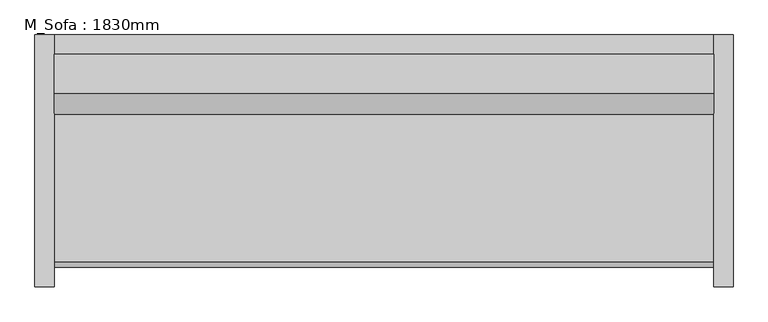
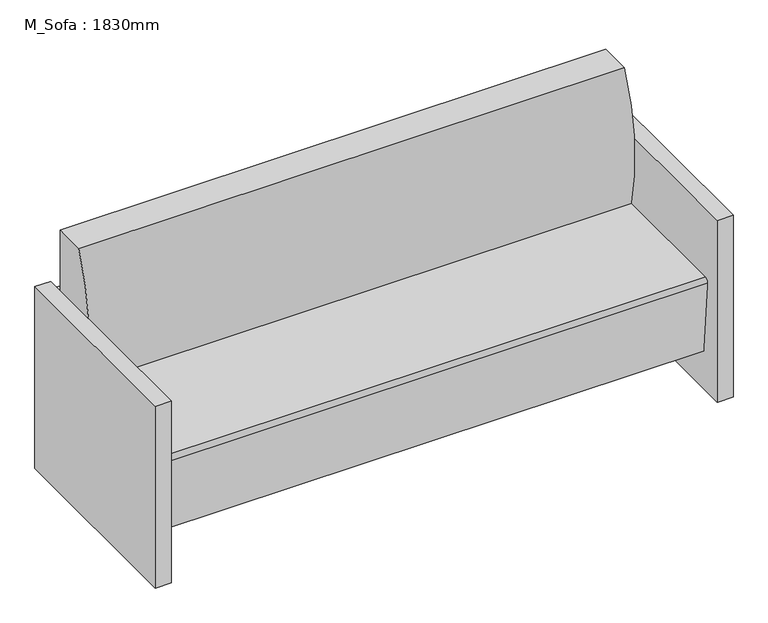
"""IFC4 building model written with IfcOpenShell, lengths in millimetres: furniture geometry, M_Sofa : 1830mm."""

from ifc_helpers import new_model, si_unit, point, frame, frame_2d, origin, origin_with_axes, place, context, project, spatial, polyline, circle_curve, trimmed, segment, composite_curve, outline, extrude, source, transform, mapped, element, save


def m_sofa_1830mm_f9e8a66b(model_context):
    return source(origin(), model_context, "Body", "SweptSolid", [
        extrude(outline(polyline([(-793.8295082, 425.5540984), (-793.8295082, 476.3540984), (934.5704918, 476.3540984), (934.5704918, 425.5540984), (-793.8295082, 425.5540984)])), frame((0.0, 0.0, 457.2), z_axis=(0.0, 0.0, 1.0), x_axis=(1.0, 0.0, 0.0)), (0.0, 0.0, 1.0), 127.0),
        extrude(outline(polyline([(-793.8295082, 425.5540984), (-793.8295082, 476.3540984), (934.5704918, 476.3540984), (934.5704918, 425.5540984), (-793.8295082, 425.5540984)])), frame((0.0, 0.0, 266.7), z_axis=(0.0, 0.0, 1.0), x_axis=(1.0, 0.0, 0.0)), (0.0, 0.0, 1.0), 127.0),
        extrude(outline(polyline([(-793.8295082, 425.5540984), (-793.8295082, 476.3540984), (934.5704918, 476.3540984), (934.5704918, 425.5540984), (-793.8295082, 425.5540984)])), frame((0.0, 0.0, 76.2), z_axis=(0.0, 0.0, 1.0), x_axis=(1.0, 0.0, 0.0)), (0.0, 0.0, 1.0), 127.0),
        extrude(outline(composite_curve([segment(trimmed(circle_curve(frame_2d((926.517198, 542.5300036)), 660.4), [point((286.1764935, 381.0))], [point((323.9540984, 812.8))], False, "CARTESIAN"), True, "CONTINUOUS"), segment(polyline([(323.9540984, 812.8), (425.5540984, 812.8), (425.5540984, 127.9665467), (-111.108343, 127.9665467), (-132.0379563, 367.1931221)]), True, "CONTINUOUS"), segment(trimmed(circle_curve(frame_2d((-119.3862837, 368.3)), 12.7), [point((-132.0379563, 367.1931221))], [point((-119.3862837, 381.0))], False, "CARTESIAN"), True, "CONTINUOUS"), segment(polyline([(-119.3862837, 381.0), (286.1764935, 381.0)]), True, "CONTINUOUS")], self_intersect=False)), frame((-793.8295082, 0.0, 0.0), z_axis=(1.0, 0.0, 0.0), x_axis=(0.0, 1.0, 0.0)), (0.0, 0.0, 1.0), 1728.4),
        extrude(outline(polyline([(-793.8295082, 476.3540984), (-793.8295082, -184.0459016), (-844.6295082, -184.0459016), (-844.6295082, 476.3540984), (-793.8295082, 476.3540984)])), origin_with_axes(), (0.0, 0.0, 1.0), 609.6),
        extrude(outline(polyline([(985.3704918, 476.3540984), (985.3704918, -184.0459016), (934.5704918, -184.0459016), (934.5704918, 476.3540984), (985.3704918, 476.3540984)])), origin_with_axes(), (0.0, 0.0, 1.0), 609.6),
    ])


if __name__ == "__main__":
    model = new_model("IFC4")
    model_context = context("Model", 3, world=origin())
    ifc_project = project(units=[si_unit("LENGTHUNIT", "METRE", prefix="MILLI")], contexts=[model_context])
    site = spatial("IfcSite", under=ifc_project)
    building = spatial("IfcBuilding", under=site)
    placement = place(None, origin())
    m_sofa_1830mm_shape = m_sofa_1830mm_f9e8a66b(model_context)
    element("IfcFurniture", 1, ObjectType="M_Sofa : 1830mm", at=placement, inside=building, context=model_context, shape_type="MappedRepresentation", body=[
        mapped(m_sofa_1830mm_shape, transform((0.0, 0.0, 0.0), x_axis=(1.0, 0.0, 0.0), y_axis=(0.0, 1.0, 0.0), z_axis=(0.0, 0.0, 1.0))),
    ])
    save(model, "model.ifc")

# Revit data of these elements
# Type "M_Sofa : 1830mm"
#   Width = 1830 mm
#   Seat Material = Linen, Beige
#   Frame Material = Cherry
#   Default Elevation = 0
# Element 1 (IfcFurniture, "M_Sofa : 1830mm")
#   Materials on its faces: "Cherry", "Linen, Beige"
# Materials
#   "Linen, Beige": class "Textile", colour RGB 249 239 230, transparency 0, Description = "Linen, beige", Cost = 0
#   "Cherry": class "Wood", colour RGB 154 107 61, transparency 0, Description = "Prunus Serotina", Cost = 0
